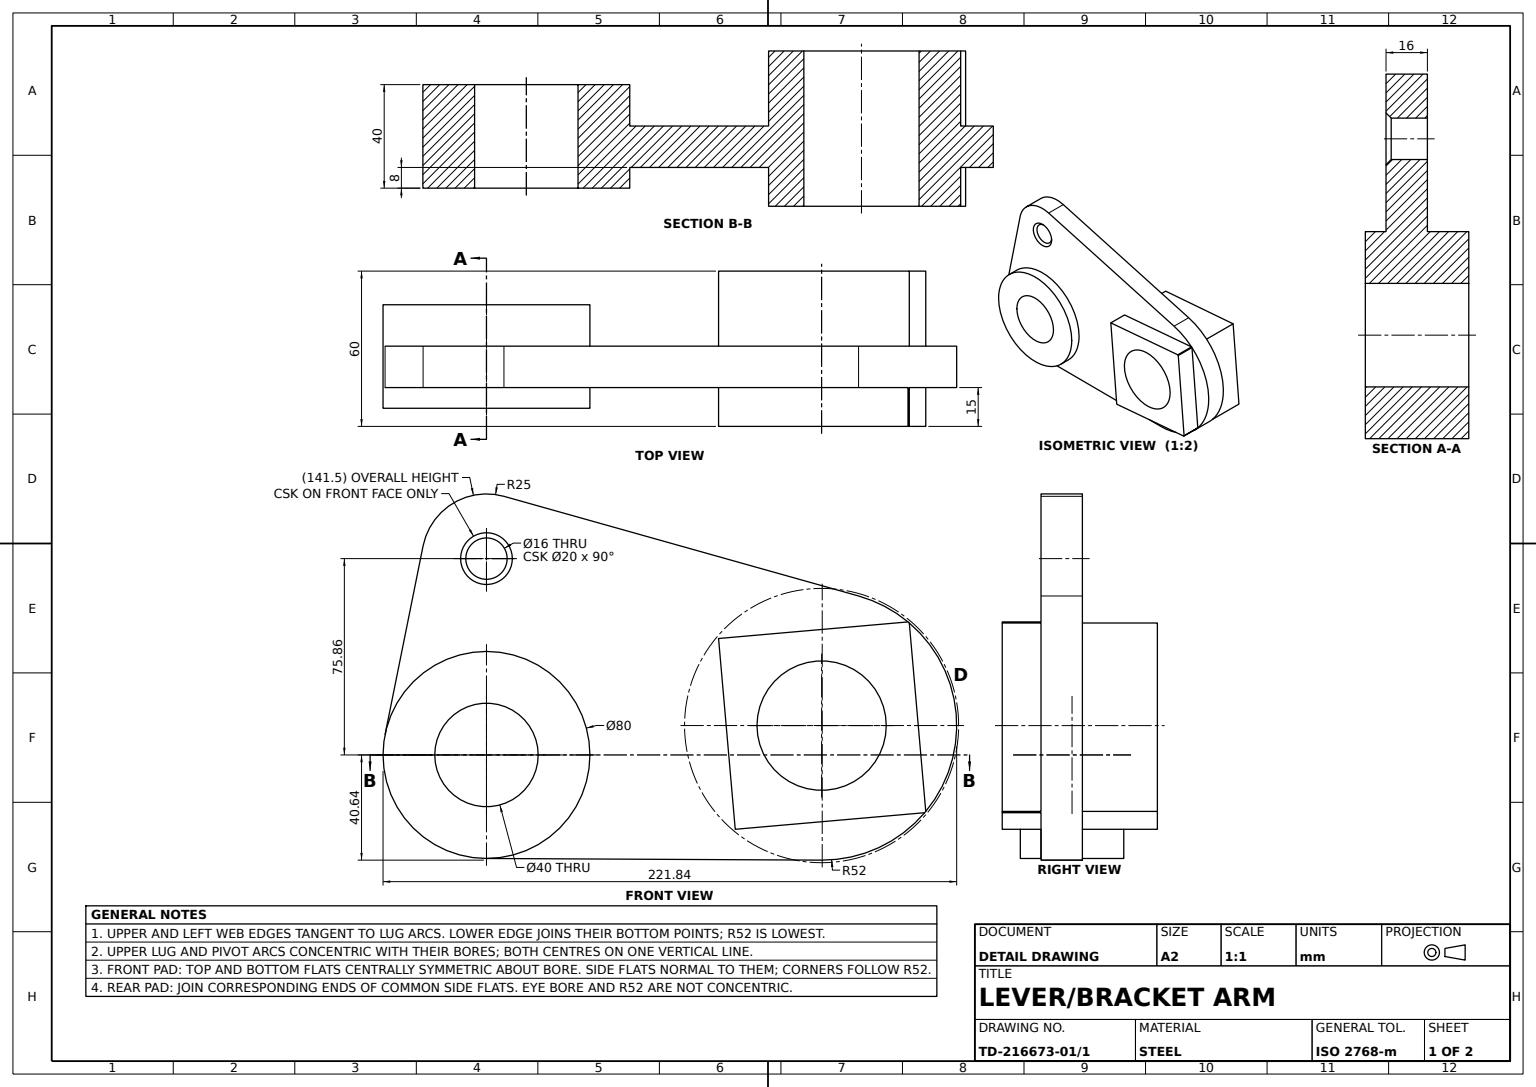
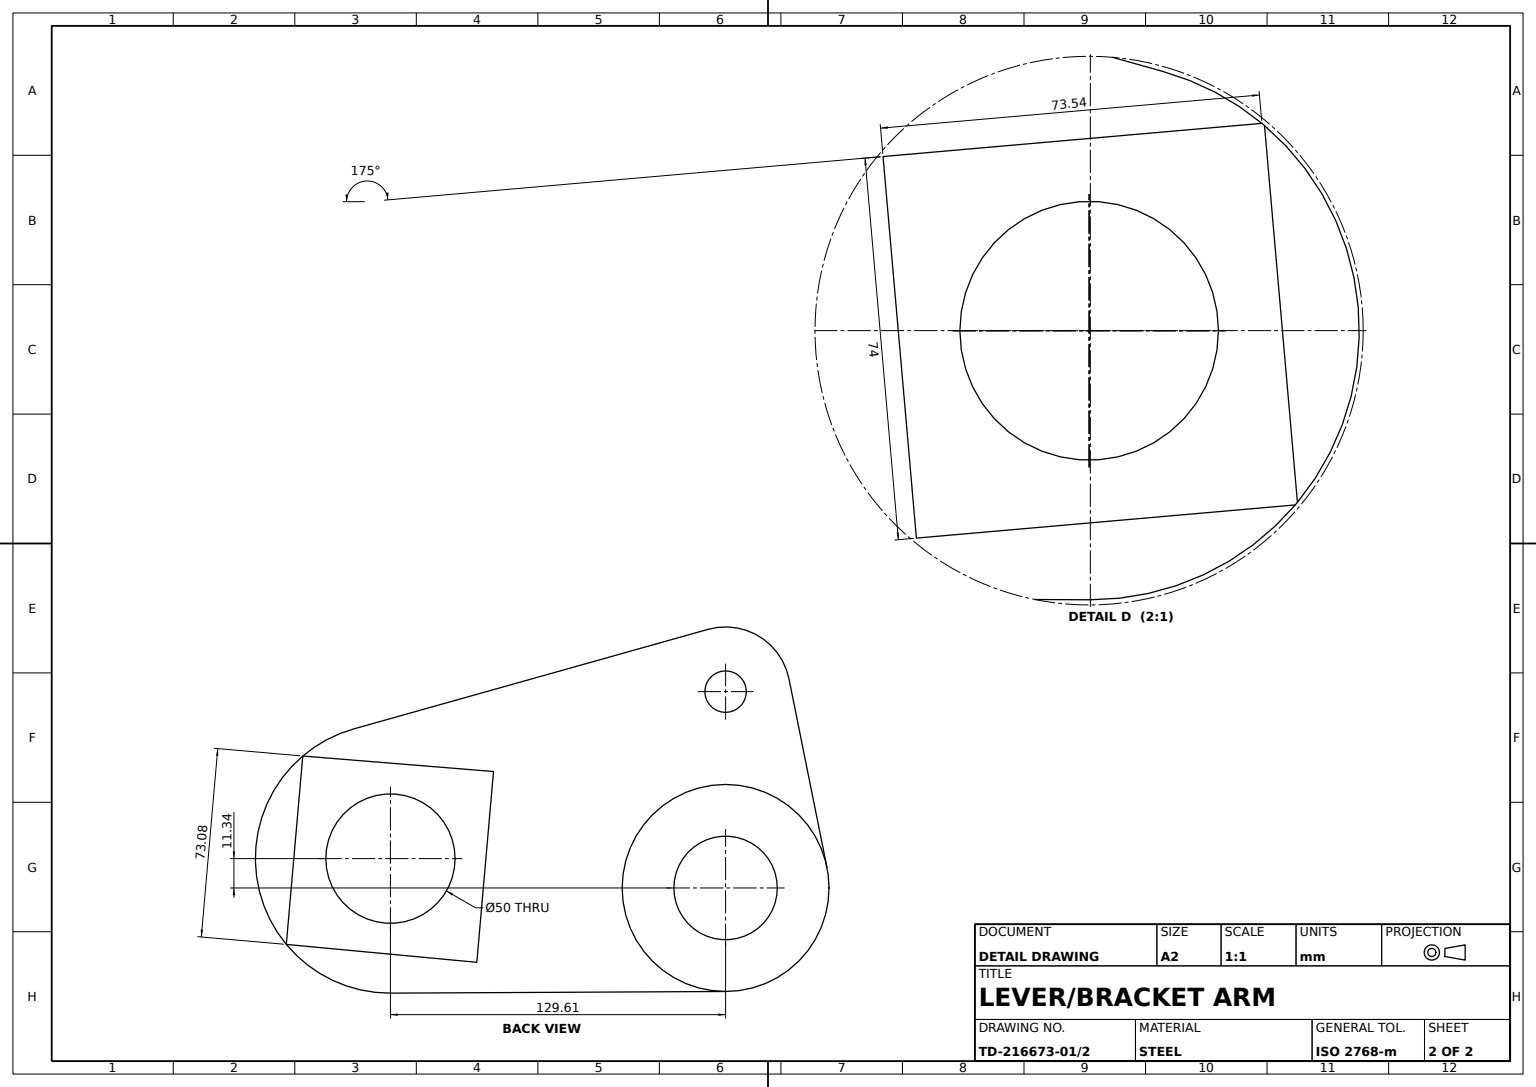
SolidWorks part; units mm, degrees
material "Plain Carbon Steel"
ref_plane "Front Plane" through (0, 0, 0) normal (0, 0, 1) x (1, 0, 0)
ref_plane "Top Plane" through (0, 0, 0) normal (0, 1, 0) x (1, 0, 0)
ref_plane "Right Plane" through (0, 0, 0) normal (1, 0, 0) x (0, 0, -1)
sketch "Lever Plate Profile" plane through (0, 0, 0) normal (0, 0, 1) x (1, 0, 0)
  line L0 (0, 0) -> (129.5, 0)
  line L1 (0, 0) -> (129.8395, 11.3595)
  line L2 (0, 0) -> (0, 75.86)
  line L3 (6.7582, 99.9292) -> (143.8965, 61.4235)
  line L4 (0, -40) -> (129.8395, -40.6405)
  line L5 (-24.5064, 80.8033) -> (-39.2102, 7.9093)
  arc A0 (-39.2102, 7.9093) -> (0, -40) centre (0, 0) ccw
  arc A1 (78.0374, 6.8274) -> (79.0954, 0) centre (129.8395, 11.3595) ccw
  arc A2 (6.7582, 99.9292) -> (-24.5064, 80.8033) centre (0, 75.86) ccw
  arc A3 (129.3265, -40.638) -> (143.8965, 61.4235) centre (129.8395, 11.3595) ccw
  dimension "D1" = 80
  dimension "D4" = 52
  dimension "D7" = 25
  dimension "D2" = 129.5
  dimension "D3" = 5
  dimension "D5" = 11.3646
  dimension "D6" = 75.86
extrude "Lever Plate" add sketch "Lever Plate Profile" along normal blind 16
sketch "Front Hub Sketch Ø40" plane through (0, 0, 16) normal (0, 0, 1) x (1, 0, 0)
  circle A0 centre (0, 0) radius 40
  dimension "D1" = 40
extrude "Front Pivot Hub Ø40" add sketch "Front Hub Sketch Ø40" along normal blind 8
sketch "Rear Hub Sketch Ø40" plane through (0, 0, 0) normal (0, 0, -1) x (-1, 0, 0)
  circle A0 centre (0, 0) radius 40
  dimension "D1" = 40
extrude "Rear Pivot Hub Ø40" add sketch "Rear Hub Sketch Ø40" along normal blind 16
sketch "Small Hole Sketch Ø8" plane through (0, 0, 16) normal (0, 0, 1) x (1, 0, 0)
  circle A0 centre (0, 75.86) radius 8
  dimension "D1" = 8
extrude "Small Hole Ø8" cut sketch "Small Hole Sketch Ø8" against normal blind 16
chamfer "Small Hole Chamfer 2mm" distance 2 angle 45 1 edges at (8, 75.86, 16)
sketch "Eye Pad Sketch 74x74" plane through (0, 0, 16) normal (0, 0, 1) x (1, 0, 0)
  line L0 (129.8395, 11.3595) -> (129.8395, 77.4524)
  line L1 (129.8395, 11.3595) -> (123.1828, 87.4463)
  line L2 (129.8395, 11.3595) -> (92.9803, 8.1347)
  line L3 (92.9803, 8.1347) -> (89.7556, 44.9939)
  line L4 (89.7556, 44.9939) -> (163.474, 51.4435)
  line L5 (163.474, 51.4435) -> (169.9235, -22.275)
  line L6 (169.9235, -22.275) -> (96.2051, -28.7245)
  line L7 (96.2051, -28.7245) -> (92.9803, 8.1347)
  arc M6 (129.8395, -40.6405) -> (143.8965, 61.4235) centre (129.8395, 11.3595) ccw
  dimension "D1" = 5
  dimension "D2" = 37
  dimension "D3" = 37
  dimension "D4" = 74
  dimension "D5" = 74
  dimension "D6" = 74
  dimension "D7" = 135.4153
  dimension "D8" = 162.393
  dimension "D9" = 202.6842
  dimension "D10" = 209.1337
  dimension "D11" = 11.916
  dimension "D12" = 118.093
extrude "Eye Pad 74x74" add sketch "Eye Pad Sketch 74x74" along normal blind 15 contours L4 L3 L2 L1 | L4 L1 L0 | L7 L6 L5 L4 L0 L2 M6
sketch "Eye Block Sketch" plane through (0, 0, 31) normal (0, 0, 1) x (1, 0, 0)
  line L0 (89.7556, 44.9939) -> (163.5143, 50.9829)
  line L1 (89.7556, 44.9939) -> (96.2051, -28.7245)
  line L2 (96.2051, -28.7245) -> (169.8832, -21.8144)
  line L3 (169.8832, -21.8144) -> (163.5143, 50.9829)
extrude "Eye Block" add sketch "Eye Block Sketch" against normal blind 60
sketch "Eye Bore Sketch Ø25" plane through (0, 0, 31) normal (0, 0, 1) x (1, 0, 0)
  line L0 (89.7556, 44.9939) -> (163.0134, 51.4032) construction
  line L1 (163.5143, 50.9829) -> (169.8832, -21.8144) construction
  circle A0 centre (129.6092, 11.3393) radius 25
  dimension "D1" = 25
  dimension "D2" = 37
  dimension "D3" = 37.2312
extrude "Eye Bore Ø25" cut sketch "Eye Bore Sketch Ø25" against normal blind 60
sketch "Pivot Bore Sketch Ø20" plane through (0, 0, 24) normal (0, 0, 1) x (1, 0, 0)
  circle A0 centre (0, 0) radius 20
  dimension "D1" = 20
extrude "Pivot Bore Ø20" cut sketch "Pivot Bore Sketch Ø20" against normal blind 40
